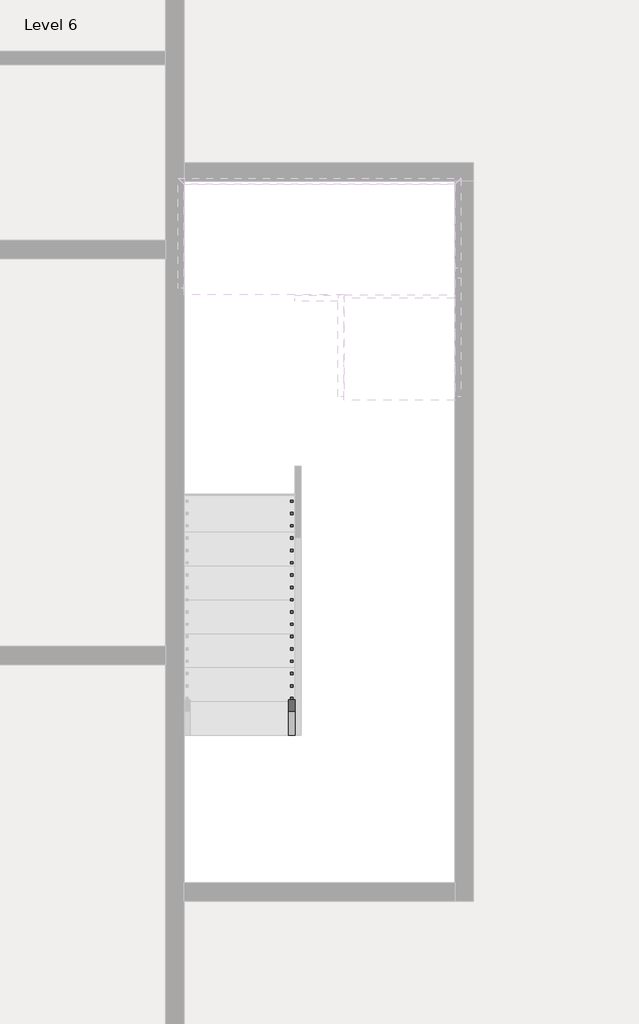
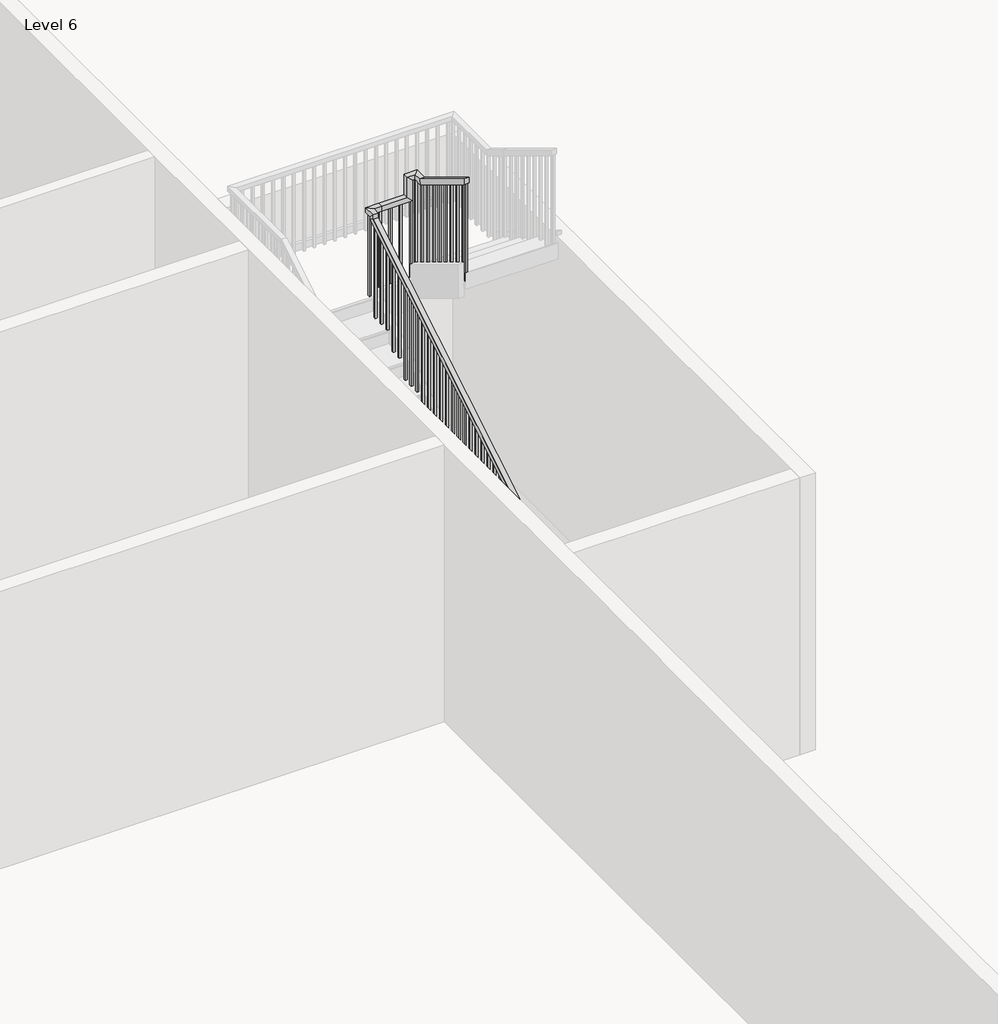
# One storey, part 5 of 8: 1 railing.
"""IFC4 building model written with IfcOpenShell, lengths in millimetres."""

from ifc_helpers import new_model, si_unit, frame, origin, place, context, project, spatial, polyline, outline, extrude, faceted_brep, element, save

model = new_model("IFC4")

# Units and contexts
model_context = context("Model", 3, world=origin())
ifc_project = project(units=[si_unit("LENGTHUNIT", "METRE", prefix="MILLI")], contexts=[model_context])

# Site, building, storey
site = spatial("IfcSite", under=ifc_project)
building = spatial("IfcBuilding", under=site)
storey = spatial("IfcBuildingStorey", under=building, Name="Level 6", Elevation=40474.6172466)

# Railing
placement = place(None, origin())
element("IfcRailing", 1, ObjectType="Handrail - Rectangular", at=placement, inside=storey, context=model_context, shape_type="SolidModel", body=[
    faceted_brep([(-2753.8415084, -23154.3851539, 41558.3505799), (-2753.8415084, -23154.3851539, 41498.9491197), (-2703.0415084, -23154.3851539, 41498.9491197), (-2703.0415084, -23154.3851539, 41558.3505799), (-2753.8415084, -19598.3851539, 43713.5020951), (-2753.8415084, -19547.5851539, 43684.8885136), (-2703.0415084, -19547.5851539, 43684.8885136), (-2703.0415084, -19598.3851539, 43713.5020951), (-2753.8415084, -19598.3851539, 43759.6839133), (-2753.8415084, -19547.5851539, 43708.8839133), (-2703.0415084, -19547.5851539, 43708.8839133), (-2703.0415084, -19598.3851539, 43759.6839133), (-2753.8415084, -19471.3851539, 43759.6839133), (-2753.8415084, -19471.3851539, 43708.8839133), (-2703.0415084, -19522.1851539, 43708.8839133), (-2703.0415084, -19522.1851539, 43759.6839133), (-2626.8415084, -19471.3851539, 43759.6839133), (-2626.8415084, -19471.3851539, 43708.8839133), (-2626.8415084, -19522.1851539, 43708.8839133), (-2626.8415084, -19522.1851539, 43759.6839133), (-2372.8415084, -19471.3851539, 43759.6839133), (-2322.0415084, -19471.3851539, 43708.8839133), (-2322.0415084, -19522.1851539, 43708.8839133), (-2372.8415084, -19522.1851539, 43759.6839133), (-2372.8415084, -19471.3851539, 43975.1990648), (-2322.0415084, -19471.3851539, 43924.3990648), (-2322.0415084, -19522.1851539, 43924.3990648), (-2372.8415084, -19522.1851539, 43975.1990648), (-2245.8415084, -19471.3851539, 43975.1990648), (-2245.8415084, -19471.3851539, 43924.3990648), (-2296.6415084, -19522.1851539, 43924.3990648), (-2296.6415084, -19522.1851539, 43975.1990648), (-2245.8415084, -19598.3851539, 43975.1990648), (-2245.8415084, -19612.5775633, 43924.3990648), (-2296.6415084, -19612.5775633, 43924.3990648), (-2296.6415084, -19598.3851539, 43975.1990648), (-2245.8415084, -20360.3851539, 44437.0172466), (-2296.6415084, -20360.3851539, 44437.0172466), (-2296.6415084, -20360.3851539, 44377.6157863), (-2245.8415084, -20360.3851539, 44377.6157863)], [[[0, 1, 2, 3]], [[1, 0, 4, 5]], [[2, 1, 5, 6]], [[3, 2, 6, 7]], [[0, 3, 7, 4]], [[5, 4, 8, 9]], [[6, 5, 9, 10]], [[7, 6, 10, 11]], [[4, 7, 11, 8]], [[9, 8, 12, 13]], [[10, 9, 13, 14]], [[11, 10, 14, 15]], [[8, 11, 15, 12]], [[13, 12, 16, 17]], [[14, 13, 17, 18]], [[15, 14, 18, 19]], [[12, 15, 19, 16]], [[17, 16, 20, 21]], [[18, 17, 21, 22]], [[19, 18, 22, 23]], [[16, 19, 23, 20]], [[21, 20, 24, 25]], [[22, 21, 25, 26]], [[23, 22, 26, 27]], [[20, 23, 27, 24]], [[25, 24, 28, 29]], [[26, 25, 29, 30]], [[27, 26, 30, 31]], [[24, 27, 31, 28]], [[29, 28, 32, 33]], [[30, 29, 33, 34]], [[31, 30, 34, 35]], [[28, 31, 35, 32]], [[36, 37, 38, 39]], [[33, 32, 36, 39]], [[34, 33, 39, 38]], [[35, 34, 38, 37]], [[32, 35, 37, 36]]]),
    extrude(outline(polyline([(-20319.1101539, 44352.6006348), (-20300.0601539, 44341.0551803), (-20300.0601539, 43353.2839133), (-20319.1101539, 43353.2839133), (-20319.1101539, 44352.6006348)])), frame((-2280.7665084, 0.0, 0.0), z_axis=(1.0, 0.0, 0.0), x_axis=(0.0, 1.0, 0.0)), (0.0, 0.0, 1.0), 19.05),
    extrude(outline(polyline([(-20217.5101539, 44291.0248773), (-20198.4601539, 44279.4794227), (-20198.4601539, 43353.2839133), (-20217.5101539, 43353.2839133), (-20217.5101539, 44291.0248773)])), frame((-2280.7665084, 0.0, 0.0), z_axis=(1.0, 0.0, 0.0), x_axis=(0.0, 1.0, 0.0)), (0.0, 0.0, 1.0), 19.05),
    extrude(outline(polyline([(-20115.9101539, 44229.4491197), (-20096.8601539, 44217.9036651), (-20096.8601539, 43353.2839133), (-20115.9101539, 43353.2839133), (-20115.9101539, 44229.4491197)])), frame((-2280.7665084, 0.0, 0.0), z_axis=(1.0, 0.0, 0.0), x_axis=(0.0, 1.0, 0.0)), (0.0, 0.0, 1.0), 19.05),
    extrude(outline(polyline([(-20014.3101539, 44167.8733621), (-19995.2601539, 44156.3279076), (-19995.2601539, 43183.9505799), (-20014.3101539, 43183.9505799), (-20014.3101539, 44167.8733621)])), frame((-2280.7665084, 0.0, 0.0), z_axis=(1.0, 0.0, 0.0), x_axis=(0.0, 1.0, 0.0)), (0.0, 0.0, 1.0), 19.05),
    extrude(outline(polyline([(-19912.7101539, 44106.2976045), (-19893.6601539, 44094.75215), (-19893.6601539, 43183.9505799), (-19912.7101539, 43183.9505799), (-19912.7101539, 44106.2976045)])), frame((-2280.7665084, 0.0, 0.0), z_axis=(1.0, 0.0, 0.0), x_axis=(0.0, 1.0, 0.0)), (0.0, 0.0, 1.0), 19.05),
    extrude(outline(polyline([(-19811.1101539, 44044.721847), (-19792.0601539, 44033.1763924), (-19792.0601539, 43183.9505799), (-19811.1101539, 43183.9505799), (-19811.1101539, 44044.721847)])), frame((-2280.7665084, 0.0, 0.0), z_axis=(1.0, 0.0, 0.0), x_axis=(0.0, 1.0, 0.0)), (0.0, 0.0, 1.0), 19.05),
    extrude(outline(polyline([(-19709.5101539, 43983.1460894), (-19690.4601539, 43971.6006348), (-19690.4601539, 43014.6172466), (-19709.5101539, 43014.6172466), (-19709.5101539, 43983.1460894)])), frame((-2280.7665084, 0.0, 0.0), z_axis=(1.0, 0.0, 0.0), x_axis=(0.0, 1.0, 0.0)), (0.0, 0.0, 1.0), 19.05),
    extrude(outline(polyline([(-19607.9101539, 43921.5703318), (-19588.8601539, 43910.0248773), (-19588.8601539, 43014.6172466), (-19607.9101539, 43014.6172466), (-19607.9101539, 43921.5703318)])), frame((-2280.7665084, 0.0, 0.0), z_axis=(1.0, 0.0, 0.0), x_axis=(0.0, 1.0, 0.0)), (0.0, 0.0, 1.0), 19.05),
    extrude(outline(polyline([(-2331.5665084, -19506.3101539), (-2331.5665084, -19487.2601539), (-2312.5165084, -19487.2601539), (-2312.5165084, -19506.3101539), (-2331.5665084, -19506.3101539)])), frame((0.0, 0.0, 42845.2839133), z_axis=(0.0, 0.0, 1.0), x_axis=(1.0, 0.0, 0.0)), (0.0, 0.0, 1.0), 1079.1151515),
    extrude(outline(polyline([(-2433.1665084, -19506.3101539), (-2433.1665084, -19487.2601539), (-2414.1165084, -19487.2601539), (-2414.1165084, -19506.3101539), (-2433.1665084, -19506.3101539)])), frame((0.0, 0.0, 42845.2839133), z_axis=(0.0, 0.0, 1.0), x_axis=(1.0, 0.0, 0.0)), (0.0, 0.0, 1.0), 863.6),
    extrude(outline(polyline([(-2534.7665084, -19506.3101539), (-2534.7665084, -19487.2601539), (-2515.7165084, -19487.2601539), (-2515.7165084, -19506.3101539), (-2534.7665084, -19506.3101539)])), frame((0.0, 0.0, 42845.2839133), z_axis=(0.0, 0.0, 1.0), x_axis=(1.0, 0.0, 0.0)), (0.0, 0.0, 1.0), 863.6),
    extrude(outline(polyline([(-2636.3665084, -19506.3101539), (-2636.3665084, -19487.2601539), (-2617.3165084, -19487.2601539), (-2617.3165084, -19506.3101539), (-2636.3665084, -19506.3101539)])), frame((0.0, 0.0, 42845.2839133), z_axis=(0.0, 0.0, 1.0), x_axis=(1.0, 0.0, 0.0)), (0.0, 0.0, 1.0), 863.6),
    extrude(outline(polyline([(-19607.9101539, 43648.3279076), (-19588.8601539, 43659.8733621), (-19588.8601539, 42675.9505799), (-19607.9101539, 42675.9505799), (-19607.9101539, 43648.3279076)])), frame((-2737.9665084, 0.0, 0.0), z_axis=(1.0, 0.0, 0.0), x_axis=(0.0, 1.0, 0.0)), (0.0, 0.0, 1.0), 19.05),
    extrude(outline(polyline([(-19709.5101539, 43586.75215), (-19690.4601539, 43598.2976045), (-19690.4601539, 42675.9505799), (-19709.5101539, 42675.9505799), (-19709.5101539, 43586.75215)])), frame((-2737.9665084, 0.0, 0.0), z_axis=(1.0, 0.0, 0.0), x_axis=(0.0, 1.0, 0.0)), (0.0, 0.0, 1.0), 19.05),
    extrude(outline(polyline([(-19811.1101539, 43525.1763924), (-19792.0601539, 43536.721847), (-19792.0601539, 42675.9505799), (-19811.1101539, 42675.9505799), (-19811.1101539, 43525.1763924)])), frame((-2737.9665084, 0.0, 0.0), z_axis=(1.0, 0.0, 0.0), x_axis=(0.0, 1.0, 0.0)), (0.0, 0.0, 1.0), 19.05),
    extrude(outline(polyline([(-19912.7101539, 43463.6006348), (-19893.6601539, 43475.1460894), (-19893.6601539, 42506.6172466), (-19912.7101539, 42506.6172466), (-19912.7101539, 43463.6006348)])), frame((-2737.9665084, 0.0, 0.0), z_axis=(1.0, 0.0, 0.0), x_axis=(0.0, 1.0, 0.0)), (0.0, 0.0, 1.0), 19.05),
    extrude(outline(polyline([(-20014.3101539, 43402.0248773), (-19995.2601539, 43413.5703318), (-19995.2601539, 42506.6172466), (-20014.3101539, 42506.6172466), (-20014.3101539, 43402.0248773)])), frame((-2737.9665084, 0.0, 0.0), z_axis=(1.0, 0.0, 0.0), x_axis=(0.0, 1.0, 0.0)), (0.0, 0.0, 1.0), 19.05),
    extrude(outline(polyline([(-20115.9101539, 43340.4491197), (-20096.8601539, 43351.9945742), (-20096.8601539, 42337.2839133), (-20115.9101539, 42337.2839133), (-20115.9101539, 43340.4491197)])), frame((-2737.9665084, 0.0, 0.0), z_axis=(1.0, 0.0, 0.0), x_axis=(0.0, 1.0, 0.0)), (0.0, 0.0, 1.0), 19.05),
    extrude(outline(polyline([(-20217.5101539, 43278.8733621), (-20198.4601539, 43290.4188166), (-20198.4601539, 42337.2839133), (-20217.5101539, 42337.2839133), (-20217.5101539, 43278.8733621)])), frame((-2737.9665084, 0.0, 0.0), z_axis=(1.0, 0.0, 0.0), x_axis=(0.0, 1.0, 0.0)), (0.0, 0.0, 1.0), 19.05),
    extrude(outline(polyline([(-20319.1101539, 43217.2976045), (-20300.0601539, 43228.8430591), (-20300.0601539, 42337.2839133), (-20319.1101539, 42337.2839133), (-20319.1101539, 43217.2976045)])), frame((-2737.9665084, 0.0, 0.0), z_axis=(1.0, 0.0, 0.0), x_axis=(0.0, 1.0, 0.0)), (0.0, 0.0, 1.0), 19.05),
    extrude(outline(polyline([(-20420.7101539, 43155.721847), (-20401.6601539, 43167.2673015), (-20401.6601539, 42167.9505799), (-20420.7101539, 42167.9505799), (-20420.7101539, 43155.721847)])), frame((-2737.9665084, 0.0, 0.0), z_axis=(1.0, 0.0, 0.0), x_axis=(0.0, 1.0, 0.0)), (0.0, 0.0, 1.0), 19.05),
    extrude(outline(polyline([(-20522.3101539, 43094.1460894), (-20503.2601539, 43105.6915439), (-20503.2601539, 42167.9505799), (-20522.3101539, 42167.9505799), (-20522.3101539, 43094.1460894)])), frame((-2737.9665084, 0.0, 0.0), z_axis=(1.0, 0.0, 0.0), x_axis=(0.0, 1.0, 0.0)), (0.0, 0.0, 1.0), 19.05),
    extrude(outline(polyline([(-20623.9101539, 43032.5703318), (-20604.8601539, 43044.1157863), (-20604.8601539, 42167.9505799), (-20623.9101539, 42167.9505799), (-20623.9101539, 43032.5703318)])), frame((-2737.9665084, 0.0, 0.0), z_axis=(1.0, 0.0, 0.0), x_axis=(0.0, 1.0, 0.0)), (0.0, 0.0, 1.0), 19.05),
    extrude(outline(polyline([(-20725.5101539, 42970.9945742), (-20706.4601539, 42982.5400288), (-20706.4601539, 41998.6172466), (-20725.5101539, 41998.6172466), (-20725.5101539, 42970.9945742)])), frame((-2737.9665084, 0.0, 0.0), z_axis=(1.0, 0.0, 0.0), x_axis=(0.0, 1.0, 0.0)), (0.0, 0.0, 1.0), 19.05),
    extrude(outline(polyline([(-20827.1101539, 42909.4188166), (-20808.0601539, 42920.9642712), (-20808.0601539, 41998.6172466), (-20827.1101539, 41998.6172466), (-20827.1101539, 42909.4188166)])), frame((-2737.9665084, 0.0, 0.0), z_axis=(1.0, 0.0, 0.0), x_axis=(0.0, 1.0, 0.0)), (0.0, 0.0, 1.0), 19.05),
    extrude(outline(polyline([(-20928.7101539, 42847.8430591), (-20909.6601539, 42859.3885136), (-20909.6601539, 41998.6172466), (-20928.7101539, 41998.6172466), (-20928.7101539, 42847.8430591)])), frame((-2737.9665084, 0.0, 0.0), z_axis=(1.0, 0.0, 0.0), x_axis=(0.0, 1.0, 0.0)), (0.0, 0.0, 1.0), 19.05),
    extrude(outline(polyline([(-21030.3101539, 42786.2673015), (-21011.2601539, 42797.812756), (-21011.2601539, 41829.2839133), (-21030.3101539, 41829.2839133), (-21030.3101539, 42786.2673015)])), frame((-2737.9665084, 0.0, 0.0), z_axis=(1.0, 0.0, 0.0), x_axis=(0.0, 1.0, 0.0)), (0.0, 0.0, 1.0), 19.05),
    extrude(outline(polyline([(-21131.9101539, 42724.6915439), (-21112.8601539, 42736.2369985), (-21112.8601539, 41829.2839133), (-21131.9101539, 41829.2839133), (-21131.9101539, 42724.6915439)])), frame((-2737.9665084, 0.0, 0.0), z_axis=(1.0, 0.0, 0.0), x_axis=(0.0, 1.0, 0.0)), (0.0, 0.0, 1.0), 19.05),
    extrude(outline(polyline([(-21233.5101539, 42663.1157863), (-21214.4601539, 42674.6612409), (-21214.4601539, 41659.9505799), (-21233.5101539, 41659.9505799), (-21233.5101539, 42663.1157863)])), frame((-2737.9665084, 0.0, 0.0), z_axis=(1.0, 0.0, 0.0), x_axis=(0.0, 1.0, 0.0)), (0.0, 0.0, 1.0), 19.05),
    extrude(outline(polyline([(-21335.1101539, 42601.5400288), (-21316.0601539, 42613.0854833), (-21316.0601539, 41659.9505799), (-21335.1101539, 41659.9505799), (-21335.1101539, 42601.5400288)])), frame((-2737.9665084, 0.0, 0.0), z_axis=(1.0, 0.0, 0.0), x_axis=(0.0, 1.0, 0.0)), (0.0, 0.0, 1.0), 19.05),
    extrude(outline(polyline([(-21436.7101539, 42539.9642712), (-21417.6601539, 42551.5097257), (-21417.6601539, 41659.9505799), (-21436.7101539, 41659.9505799), (-21436.7101539, 42539.9642712)])), frame((-2737.9665084, 0.0, 0.0), z_axis=(1.0, 0.0, 0.0), x_axis=(0.0, 1.0, 0.0)), (0.0, 0.0, 1.0), 19.05),
    extrude(outline(polyline([(-21538.3101539, 42478.3885136), (-21519.2601539, 42489.9339682), (-21519.2601539, 41490.6172466), (-21538.3101539, 41490.6172466), (-21538.3101539, 42478.3885136)])), frame((-2737.9665084, 0.0, 0.0), z_axis=(1.0, 0.0, 0.0), x_axis=(0.0, 1.0, 0.0)), (0.0, 0.0, 1.0), 19.05),
    extrude(outline(polyline([(-21639.9101539, 42416.812756), (-21620.8601539, 42428.3582106), (-21620.8601539, 41490.6172466), (-21639.9101539, 41490.6172466), (-21639.9101539, 42416.812756)])), frame((-2737.9665084, 0.0, 0.0), z_axis=(1.0, 0.0, 0.0), x_axis=(0.0, 1.0, 0.0)), (0.0, 0.0, 1.0), 19.05),
    extrude(outline(polyline([(-21741.5101539, 42355.2369985), (-21722.4601539, 42366.782453), (-21722.4601539, 41490.6172466), (-21741.5101539, 41490.6172466), (-21741.5101539, 42355.2369985)])), frame((-2737.9665084, 0.0, 0.0), z_axis=(1.0, 0.0, 0.0), x_axis=(0.0, 1.0, 0.0)), (0.0, 0.0, 1.0), 19.05),
    extrude(outline(polyline([(-21843.1101539, 42293.6612409), (-21824.0601539, 42305.2066954), (-21824.0601539, 41321.2839133), (-21843.1101539, 41321.2839133), (-21843.1101539, 42293.6612409)])), frame((-2737.9665084, 0.0, 0.0), z_axis=(1.0, 0.0, 0.0), x_axis=(0.0, 1.0, 0.0)), (0.0, 0.0, 1.0), 19.05),
    extrude(outline(polyline([(-21944.7101539, 42232.0854833), (-21925.6601539, 42243.6309379), (-21925.6601539, 41321.2839133), (-21944.7101539, 41321.2839133), (-21944.7101539, 42232.0854833)])), frame((-2737.9665084, 0.0, 0.0), z_axis=(1.0, 0.0, 0.0), x_axis=(0.0, 1.0, 0.0)), (0.0, 0.0, 1.0), 19.05),
    extrude(outline(polyline([(-22046.3101539, 42170.5097257), (-22027.2601539, 42182.0551803), (-22027.2601539, 41321.2839133), (-22046.3101539, 41321.2839133), (-22046.3101539, 42170.5097257)])), frame((-2737.9665084, 0.0, 0.0), z_axis=(1.0, 0.0, 0.0), x_axis=(0.0, 1.0, 0.0)), (0.0, 0.0, 1.0), 19.05),
    extrude(outline(polyline([(-22147.9101539, 42108.9339682), (-22128.8601539, 42120.4794227), (-22128.8601539, 41151.9505799), (-22147.9101539, 41151.9505799), (-22147.9101539, 42108.9339682)])), frame((-2737.9665084, 0.0, 0.0), z_axis=(1.0, 0.0, 0.0), x_axis=(0.0, 1.0, 0.0)), (0.0, 0.0, 1.0), 19.05),
    extrude(outline(polyline([(-22249.5101539, 42047.3582106), (-22230.4601539, 42058.9036651), (-22230.4601539, 41151.9505799), (-22249.5101539, 41151.9505799), (-22249.5101539, 42047.3582106)])), frame((-2737.9665084, 0.0, 0.0), z_axis=(1.0, 0.0, 0.0), x_axis=(0.0, 1.0, 0.0)), (0.0, 0.0, 1.0), 19.05),
    extrude(outline(polyline([(-22351.1101539, 41985.782453), (-22332.0601539, 41997.3279076), (-22332.0601539, 40982.6172466), (-22351.1101539, 40982.6172466), (-22351.1101539, 41985.782453)])), frame((-2737.9665084, 0.0, 0.0), z_axis=(1.0, 0.0, 0.0), x_axis=(0.0, 1.0, 0.0)), (0.0, 0.0, 1.0), 19.05),
    extrude(outline(polyline([(-22452.7101539, 41924.2066954), (-22433.6601539, 41935.75215), (-22433.6601539, 40982.6172466), (-22452.7101539, 40982.6172466), (-22452.7101539, 41924.2066954)])), frame((-2737.9665084, 0.0, 0.0), z_axis=(1.0, 0.0, 0.0), x_axis=(0.0, 1.0, 0.0)), (0.0, 0.0, 1.0), 19.05),
    extrude(outline(polyline([(-22554.3101539, 41862.6309379), (-22535.2601539, 41874.1763924), (-22535.2601539, 40982.6172466), (-22554.3101539, 40982.6172466), (-22554.3101539, 41862.6309379)])), frame((-2737.9665084, 0.0, 0.0), z_axis=(1.0, 0.0, 0.0), x_axis=(0.0, 1.0, 0.0)), (0.0, 0.0, 1.0), 19.05),
    extrude(outline(polyline([(-22655.9101539, 41801.0551803), (-22636.8601539, 41812.6006348), (-22636.8601539, 40813.2839133), (-22655.9101539, 40813.2839133), (-22655.9101539, 41801.0551803)])), frame((-2737.9665084, 0.0, 0.0), z_axis=(1.0, 0.0, 0.0), x_axis=(0.0, 1.0, 0.0)), (0.0, 0.0, 1.0), 19.05),
    extrude(outline(polyline([(-22757.5101539, 41739.4794227), (-22738.4601539, 41751.0248773), (-22738.4601539, 40813.2839133), (-22757.5101539, 40813.2839133), (-22757.5101539, 41739.4794227)])), frame((-2737.9665084, 0.0, 0.0), z_axis=(1.0, 0.0, 0.0), x_axis=(0.0, 1.0, 0.0)), (0.0, 0.0, 1.0), 19.05),
    extrude(outline(polyline([(-22859.1101539, 41677.9036651), (-22840.0601539, 41689.4491197), (-22840.0601539, 40813.2839133), (-22859.1101539, 40813.2839133), (-22859.1101539, 41677.9036651)])), frame((-2737.9665084, 0.0, 0.0), z_axis=(1.0, 0.0, 0.0), x_axis=(0.0, 1.0, 0.0)), (0.0, 0.0, 1.0), 19.05),
    extrude(outline(polyline([(-22960.7101539, 41616.3279076), (-22941.6601539, 41627.8733621), (-22941.6601539, 40643.9505799), (-22960.7101539, 40643.9505799), (-22960.7101539, 41616.3279076)])), frame((-2737.9665084, 0.0, 0.0), z_axis=(1.0, 0.0, 0.0), x_axis=(0.0, 1.0, 0.0)), (0.0, 0.0, 1.0), 19.05),
    extrude(outline(polyline([(-23062.3101539, 41554.75215), (-23043.2601539, 41566.2976045), (-23043.2601539, 40643.9505799), (-23062.3101539, 40643.9505799), (-23062.3101539, 41554.75215)])), frame((-2737.9665084, 0.0, 0.0), z_axis=(1.0, 0.0, 0.0), x_axis=(0.0, 1.0, 0.0)), (0.0, 0.0, 1.0), 19.05),
    extrude(outline(polyline([(-2280.7665084, -19506.3101539), (-2280.7665084, -19487.2601539), (-2261.7165084, -19487.2601539), (-2261.7165084, -19506.3101539), (-2280.7665084, -19506.3101539)])), frame((0.0, 0.0, 42845.2839133), z_axis=(0.0, 0.0, 1.0), x_axis=(1.0, 0.0, 0.0)), (0.0, 0.0, 1.0), 1079.1151515),
    extrude(outline(polyline([(-2718.9165084, -19506.3101539), (-2737.9665084, -19506.3101539), (-2737.9665084, -19487.2601539), (-2718.9165084, -19487.2601539), (-2718.9165084, -19506.3101539)])), frame((0.0, 0.0, 42845.2839133), z_axis=(0.0, 0.0, 1.0), x_axis=(1.0, 0.0, 0.0)), (0.0, 0.0, 1.0), 863.6),
    extrude(outline(polyline([(-20360.3851539, 44377.6157863), (-20341.3351539, 44366.0703318), (-20341.3351539, 43353.2839133), (-20360.3851539, 43353.2839133), (-20360.3851539, 44377.6157863)])), frame((-2280.7665084, 0.0, 0.0), z_axis=(1.0, 0.0, 0.0), x_axis=(0.0, 1.0, 0.0)), (0.0, 0.0, 1.0), 19.05),
    extrude(outline(polyline([(-23154.3851539, 41498.9491197), (-23135.3351539, 41510.4945742), (-23135.3351539, 40643.9505799), (-23154.3851539, 40643.9505799), (-23154.3851539, 41498.9491197)])), frame((-2737.9665084, 0.0, 0.0), z_axis=(1.0, 0.0, 0.0), x_axis=(0.0, 1.0, 0.0)), (0.0, 0.0, 1.0), 19.05),
])

save(model, "model.ifc")

# Revit data of these elements
# Type "Handrail - Rectangular"
#   Assembly Code = "C2010400"
#   built-in parameter 1008612 = 0.0416667 (stored number, unit not read)
#   built-in parameter 1008611 = 0.0416667 (stored number, unit not read)
#   built-in parameter 1008609 = 0.333333 (stored number, unit not read)
#   built-in parameter 1008604 = 0.166667 (stored number, unit not read)
#   built-in parameter 1008603 = 0.166667 (stored number, unit not read)
#   Railing Height = 3' - 0"
#   built-in parameter 1008630 = 2
#   built-in parameter 1008610 = 2
#   built-in parameter 1008618 = Baluster - Square : 3/4"
# Element 1 (IfcRailing, "Handrail - Rectangular")
#   Phase Created = New Construction
